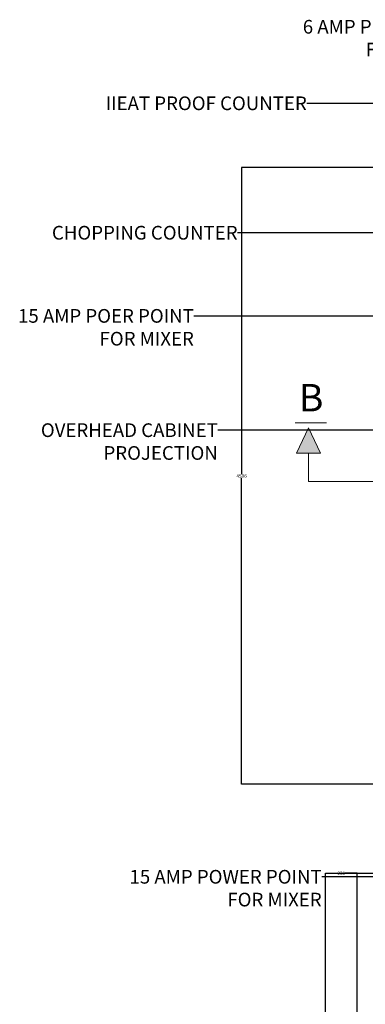
# Model space of a CAD drawing. Units: millimetres. Extents: x 1944 to 29915, y -10550 to 5909.
# Tile 2 of 24: x 4181 to 6709, y -1353 to 5842. Entities that reach past the tile are written whole.
import ezdxf
from ezdxf import colors
from ezdxf.entities.mleader import LeaderData, LeaderLine
from ezdxf.math import Vec2, Vec3

# ---------------------------------------------------------------- set-up
doc = ezdxf.new("R2010")
doc.units = ezdxf.units.MM
doc.header["$MEASUREMENT"] = 0
for name, color, linetype, lineweight in [('A-ANNO-DIMS', 2, 'Continuous', 18), ('A-ANNO-SYMB', 2, 'Continuous', 18), ('A-ANNO-TEXT', 7, 'Continuous', 25)]:
    doc.layers.add(name, color=color, linetype=linetype, lineweight=lineweight)
doc.styles.get("Standard").update_dxf_attribs({"font": 'arial.ttf'})
doc.dimstyles.get("Standard").update_dxf_attribs({"dimtxt": 25, "dimasz": 0.18, "dimexe": 0.18, "dimexo": 0.0625, "dimgap": 0.09, "dimtad": 0, "dimtih": 1, "dimtoh": 1, "dimdec": 0, "dimzin": 0, "dimdsep": 46, "dimtxsty": 'Standard', "dimcen": 0.09, "dimadec": 0, "dimazin": 0, "dimtfac": 1, "dimtdec": 0, "dimtofl": 0, "dimtmove": 0, "dimatfit": 3, "dimfxl": 1, "dimtolj": 1, "dimtzin": 0, "dimarcsym": 0})

# ---------------------------------------------------------------- blocks, each defined once
blk = doc.blocks.new('*D57')
at = {"layer": 'A-ANNO-DIMS', "color": 0, "lineweight": -2, "transparency": 16777216}
for p, q in [((8995.2, 4760.8), (5803.8, 4760.8)), ((5804, 4760.7), (5804, 2520.7)), ((5804, 255), (5804, 2495)), ((8999.6, 254.8), (5803.8, 254.8))]:
    blk.add_line(p, q, dxfattribs=at)
at = {"layer": 'A-ANNO-DIMS', "color": 0, "transparency": 16777216}
for points in [[(5804, 4760.7), (5804, 4760.7), (5804, 4760.8)], [(5804, 255), (5804, 255), (5804, 254.8)]]:
    blk.add_solid(points, dxfattribs=at)
at = {"layer": 'Defpoints', "color": 0, "transparency": 16777216}
for p in [(8995.2, 4760.8), (5804, 254.8), (8999.6, 254.8)]:
    blk.add_point(p, dxfattribs=at)
at = {"layer": 'A-ANNO-DIMS', "color": 0, "transparency": 16777216, "insert": (5804, 2507.8), "char_height": 25, "attachment_point": 5}
blk.add_mtext('\\A1;4506', dxfattribs=at)
blk = doc.blocks.new('*D85')
at = {"layer": 'A-ANNO-DIMS', "color": 0, "lineweight": -2, "transparency": 16777216}
for p, q in [((6418.3, -1730.7), (6418.3, -395.6)), ((6418.5, -395.8), (15860.3, -395.8)), ((25389.1, -395.8), (15947.3, -395.8)), ((25389.3, -1846.5), (25389.3, -395.6))]:
    blk.add_line(p, q, dxfattribs=at)
at = {"layer": 'A-ANNO-DIMS', "color": 0, "transparency": 16777216}
for points in [[(6418.5, -395.7), (6418.5, -395.8), (6418.3, -395.8)], [(25389.1, -395.7), (25389.1, -395.8), (25389.3, -395.8)]]:
    blk.add_solid(points, dxfattribs=at)
at = {"layer": 'Defpoints', "color": 0, "transparency": 16777216}
for p in [(25389.3, -395.8), (6418.3, -1730.8), (25389.3, -1846.5)]:
    blk.add_point(p, dxfattribs=at)
at = {"layer": 'A-ANNO-DIMS', "color": 0, "transparency": 16777216, "insert": (15903.8, -395.8), "char_height": 25, "attachment_point": 5}
blk.add_mtext('\\A1;18971', dxfattribs=at)
blk = doc.blocks.new('*D90')
at = {"layer": 'A-ANNO-DIMS', "color": 0, "lineweight": -2, "transparency": 16777216}
for p, q in [((6418.3, -3019.9), (6418.3, -395.6)), ((6418.5, -395.8), (6505.4, -395.8)), ((6648.1, -395.8), (6561.2, -395.8)), ((6648.3, -3075.9), (6648.3, -395.6))]:
    blk.add_line(p, q, dxfattribs=at)
at = {"layer": 'A-ANNO-DIMS', "color": 0, "transparency": 16777216}
for points in [[(6418.5, -395.7), (6418.5, -395.8), (6418.3, -395.8)], [(6648.1, -395.7), (6648.1, -395.8), (6648.3, -395.8)]]:
    blk.add_solid(points, dxfattribs=at)
at = {"layer": 'Defpoints', "color": 0, "transparency": 16777216}
for p in [(6648.3, -395.8), (6418.3, -3020), (6648.3, -3076)]:
    blk.add_point(p, dxfattribs=at)
at = {"layer": 'A-ANNO-DIMS', "color": 0, "transparency": 16777216, "insert": (6533.3, -395.8), "char_height": 25, "attachment_point": 5}
blk.add_mtext('\\A1;230', dxfattribs=at)

msp = doc.modelspace()

# ---------------------------------------------------------------- hatches: boundary and pattern name
at = {"layer": 'A-ANNO-SYMB'}
h = msp.add_hatch(color=256, dxfattribs=at)
h.dxf.hatch_style = 1
h.paths.add_polyline_path([(6293.436, 2859.206), (6205.406, 2673.669), (6293.436, 2673.669), (6381.467, 2673.669)])

# ---------------------------------------------------------------- linework, layer by layer
for p, q in [((6196.234, 2896.746), (6424.724, 2896.746)), ((6205.406, 2673.669), (6293.436, 2859.206)), ((6381.467, 2673.669), (6293.436, 2859.206)), ((6293.436, 2673.669), (6205.406, 2673.669)), ((6293.436, 2468.085), (6293.436, 2673.669)), ((6293.436, 2673.669), (6381.467, 2673.669)), ((6293.436, 2468.085), (10483.966, 2468.085))]:
    msp.add_line(p, q, dxfattribs=at)

# ---------------------------------------------------------------- texts
at = {"layer": 'A-ANNO-TEXT'}
msp.add_text('B', height=200, dxfattribs=at).set_placement((6222.981, 2979.554))

# ---------------------------------------------------------------- dimensions: what is measured, and where the dimension line sits
at = {"layer": 'A-ANNO-DIMS'}
dim = msp.add_linear_dim(base=(5803.984, 254.791), p1=(8995.217, 4760.837), p2=(8999.621, 254.791), angle=90, dimstyle='Standard', override={"dimdec": 0, "dimlfac": 1, "dimrnd": 0, "dimzin": 0, "dimdsep": 46, "dimlunit": 2}, dxfattribs=at)
dim.commit()
dim.dimension.update_dxf_attribs({"geometry": '*D57', "text_midpoint": (5803.984, 2507.814)})
for base, p1, p2, picture, middle in [((25389.297, -395.752), (6418.315, -1730.752), (25389.297, -1846.542), '*D85', (15903.806, -395.752)), ((6648.315, -395.752), (6418.315, -3019.985), (6648.315, -3075.967), '*D90', (6533.315, -395.752))]:
    dim = msp.add_linear_dim(base=base, p1=p1, p2=p2, dimstyle='Standard', override={"dimdec": 0, "dimlfac": 1, "dimrnd": 0, "dimzin": 0, "dimdsep": 46, "dimlunit": 2}, dxfattribs=at)
    dim.commit()
    dim.dimension.update_dxf_attribs({"geometry": picture, "text_midpoint": middle})

# ---------------------------------------------------------------- leaders
at = {"layer": 'A-ANNO-TEXT'}
ml = msp.add_multileader_mtext('Standard', dxfattribs=at)
ml.set_content('6 AMP PLUG POINT\\PFOR EX.FAN ', color=256)
ml.set_leader_properties()
ml.build(insert=Vec2(0, 0))
ml.multileader.update_dxf_attribs({"dogleg_length": 568.936, "arrow_head_size": 100})
ctx = ml.context
ctx.base_point, ctx.char_height, ctx.arrow_head_size, ctx.landing_gap_size, ctx.plane_origin = Vec3(6163.428, 5789.061), 100, 100, 0.09, Vec3(7359.519, 5416.773)
ctx.text_align_type = 2
notes = []
notes.append((ctx, [(0, (1, 1, 0), (8028.655, 5789.061), (-1, 0), 568.936, [(0, [(8031.498, 4870.48), (8028.655, 5789.061)], 0, [])])]))
ctx.mtext.insert, ctx.mtext.alignment, ctx.mtext.flow_direction = Vec3(7459.63, 5839.914), 3, 5
ml = msp.add_multileader_mtext('Standard', dxfattribs=at)
ml.set_content('IIEAT PROOF COUNTER', color=256)
ml.set_leader_properties()
ml.build(insert=Vec2(0, 0))
ml.multileader.update_dxf_attribs({"dogleg_length": 568.936, "arrow_head_size": 100})
ctx = ml.context
ctx.base_point, ctx.char_height, ctx.arrow_head_size, ctx.landing_gap_size, ctx.plane_origin = Vec3(4680.871, 5230.05), 100, 100, 0.09, Vec3(6849.578, 5230.05)
ctx.text_align_type = 2
notes.append((ctx, [(0, (1, 1, 0), (6849.578, 5230.05), (-1, 0), 568.936, [(0, [(7225.221, 4609.585), (7225.221, 5230.05)], 0, [])])]))
ctx.mtext.insert, ctx.mtext.alignment, ctx.mtext.flow_direction = Vec3(6280.552, 5280.903), 3, 5
ml = msp.add_multileader_mtext('Standard', dxfattribs=at)
ml.set_content('CHOPPING COUNTER', color=256)
ml.set_leader_properties()
ml.build(insert=Vec2(0, 0))
ml.multileader.update_dxf_attribs({"dogleg_length": 568.936, "arrow_head_size": 100})
ctx = ml.context
ctx.base_point, ctx.char_height, ctx.arrow_head_size, ctx.landing_gap_size, ctx.plane_origin = Vec3(4308.291, 4284.103), 100, 100, 0.09, Vec3(6343.369, 4284.103)
ctx.text_align_type = 2
notes.append((ctx, [(0, (1, 1, 0), (6343.369, 4284.103), (-1, 0), 568.936, [(0, [(7137.476, 4280.213), (7137.476, 4284.103)], 0, [])])]))
ctx.mtext.insert, ctx.mtext.alignment, ctx.mtext.flow_direction = Vec3(5774.343, 4334.955), 3, 5
ml = msp.add_multileader_mtext('Standard', dxfattribs=at)
ml.set_content('15 AMP POER POINT \\PFOR MIXER', color=256)
ml.set_leader_properties()
ml.build(insert=Vec2(0, 0))
ml.multileader.update_dxf_attribs({"dogleg_length": 568.936, "arrow_head_size": 100})
ctx = ml.context
ctx.base_point, ctx.char_height, ctx.arrow_head_size, ctx.landing_gap_size, ctx.plane_origin = Vec3(4075.208, 3676.447), 100, 100, 0.09, Vec3(6023.655, 3676.447)
ctx.text_align_type = 2
notes.append((ctx, [(0, (1, 1, 0), (6023.655, 3676.447), (-1, 0), 568.936, [(0, [(6929.507, 3676.447), (6937.725, 3676.447)], 0, [])])]))
ctx.mtext.insert, ctx.mtext.alignment, ctx.mtext.flow_direction = Vec3(5454.629, 3727.299), 3, 5
ml = msp.add_multileader_mtext('Standard', dxfattribs=at)
ml.set_content('OVERHEAD CABINET \\PPROJECTION', color=256)
ml.set_leader_properties()
ml.build(insert=Vec2(0, 0))
ml.multileader.update_dxf_attribs({"dogleg_length": 568.936, "arrow_head_size": 100})
ctx = ml.context
ctx.base_point, ctx.char_height, ctx.arrow_head_size, ctx.landing_gap_size, ctx.plane_origin = Vec3(4211.068, 2841.398), 100, 100, 0.09, Vec3(6198.942, 2841.398)
ctx.text_align_type = 2
notes.append((ctx, [(0, (1, 1, 0), (6198.942, 2841.398), (-1, 0), 568.936, [(0, [(7130.068, 2828.866), (7130.068, 2841.398)], 0, [])])]))
ctx.mtext.insert, ctx.mtext.alignment, ctx.mtext.flow_direction = Vec3(5629.917, 2892.251), 3, 5
ml = msp.add_multileader_mtext('Standard', dxfattribs=at)
ml.set_content('15 AMP POWER POINT \\PFOR MIXER', color=256)
ml.set_leader_properties()
ml.build(insert=Vec2(0, 0))
ml.multileader.update_dxf_attribs({"dogleg_length": 568.936, "arrow_head_size": 100})
ctx = ml.context
ctx.base_point, ctx.char_height, ctx.arrow_head_size, ctx.landing_gap_size, ctx.plane_origin = Vec3(4878.252, -422.117), 100, 100, 0.09, Vec3(6870.097, -798.764)
ctx.text_align_type = 2
notes.append((ctx, [(0, (1, 1, 0), (6958.555, -422.117), (-1, 0), 568.936, [(0, [(8384.052, 260.837), (8397.606, -446.246)], 0, [])])]))
ctx.mtext.insert, ctx.mtext.alignment, ctx.mtext.flow_direction = Vec3(6389.529, -371.264), 3, 5
for ctx, leaders in notes:
    for number, flags, end, landing, length, lines in leaders:
        leader = LeaderData()
        leader.index, (leader.has_last_leader_line, leader.has_dogleg_vector, leader.attachment_direction) = number, flags
        leader.last_leader_point, leader.dogleg_vector, leader.dogleg_length = Vec3(end), Vec3(landing), length
        for number, points, colour, breaks in lines:
            line = LeaderLine()
            line.index, line.vertices, line.color, line.breaks = number, Vec3.list(points), colors.encode_raw_color(colour), breaks
            leader.lines.append(line)
        ctx.leaders.append(leader)

doc.saveas('drawing.dxf')
